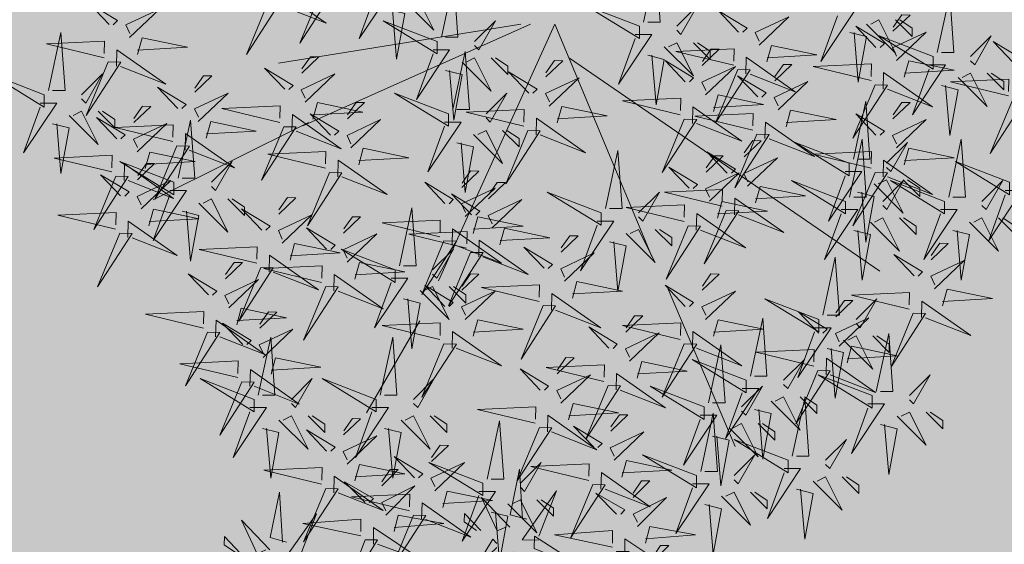
# Model space of a CAD drawing. Units: inches. Extents: x 1704 to 6393, y -157 to 1172.
# Tile 112 of 122: x 2688 to 2716, y 1003 to 1018. Entities that reach past the tile are written whole.
import ezdxf

# ---------------------------------------------------------------- set-up
doc = ezdxf.new("R2010")
doc.units = ezdxf.units.IN
doc.header["$MEASUREMENT"] = 0
doc.layers.add('A-ANNO-DIMS', color=7, linetype='Continuous', lineweight=13)
doc.layers.add('L-shrub', color=74, linetype='Continuous', lineweight=18)
doc.layers.add('L-HRDS-PATT', color=9, linetype='Continuous', lineweight=13, true_color=0xc5c1ba)
doc.styles.get("Standard").update_dxf_attribs({"font": 'arial.ttf'})
doc.dimstyles.get("Standard").update_dxf_attribs({"dimtxt": 6, "dimasz": 2, "dimexe": 0.18, "dimexo": 0.0625, "dimgap": 0.09, "dimtad": 0, "dimtih": 1, "dimtoh": 1, "dimdec": 1, "dimzin": 0, "dimdsep": 46, "dimlunit": 3, "dimtxsty": 'Standard', "dimblk": 'ARCHTICK', "dimcen": 0.09, "dimadec": 0, "dimazin": 0, "dimtfac": 1, "dimtdec": 1, "dimtofl": 0, "dimtmove": 0, "dimatfit": 3, "dimfxl": 1, "dimtolj": 1, "dimtzin": 0, "dimarcsym": 0})

# ---------------------------------------------------------------- blocks, each defined once
blk = doc.blocks.new('shrub3')
for p, q in [((-68.47, 143.52), (-106.19, 232.32)), ((68.94, 162.35), (98.58, 213.48)), ((-5.99, -2.5), (58.67, 140.12)), ((-14.08, 16.34), (-186.51, 134.74)), ((-5.99, -2.5), (-59.88, 126.66)), ((130.91, 52.02), (217.13, 95.08)), ((7.48, -2.5), (134.11, 54.01)), ((12.87, -2.5), (147.58, 19.03))]:
    blk.add_line(p, q)
for points in [[(29.32, 268.76), (20.08, 271.07), (24.7, 296.43), (27.01, 268.76)], [(72.58, 270.39), (84.86, 300.11), (65.67, 270.57), (72.58, 270.39)], [(-89.4, 264.53), (-98.64, 266.83), (-94.02, 292.2), (-91.71, 264.53)], [(36.24, 257.23), (27.01, 257.23), (45.48, 284.9), (36.24, 259.54)], [(121.34, 255.57), (133.62, 285.29), (114.43, 255.75), (121.34, 255.57)], [(-140.28, 256.06), (-149.52, 258.36), (-144.9, 283.73), (-142.59, 256.06)], [(-82.48, 253), (-91.71, 253), (-73.24, 280.67), (-82.48, 255.31)], [(-27.06, 253.45), (-14.78, 283.17), (-33.97, 253.63), (-27.06, 253.45)], [(20.08, 264.15), (3.92, 280.29), (13.16, 261.85), (17.78, 264.15)], [(68.03, 272.82), (67.8, 263.59), (40.6, 282.74), (65.73, 272.87)], [(-98.64, 259.92), (-114.8, 276.06), (-105.56, 257.61), (-100.94, 259.92)], [(-133.36, 244.53), (-142.59, 244.53), (-124.12, 272.2), (-133.36, 246.84)], [(3.92, 261.85), (-5.31, 271.07), (-5.31, 266.46), (1.62, 261.85)], [(-149.52, 251.45), (-165.68, 267.59), (-156.44, 249.14), (-151.83, 251.45)], [(-114.8, 257.61), (-124.03, 266.83), (-124.03, 262.22), (-117.11, 257.61)], [(-31.61, 255.88), (-31.84, 246.65), (-59.04, 265.8), (-33.91, 255.94)], [(56.33, 266.18), (53.8, 257.01), (28.56, 262.26), (56.27, 263.87)], [(74.83, 268.03), (106.93, 260.3), (74.6, 258.8), (74.77, 265.72)], [(116.79, 258), (116.56, 248.76), (89.36, 267.92), (114.49, 258.05)], [(-165.68, 249.14), (-174.91, 258.36), (-174.91, 253.75), (-167.99, 249.14)], [(13.16, 252.62), (1.62, 241.09), (10.85, 257.23), (13.16, 254.93)], [(33.94, 252.62), (63.95, 241.09), (33.94, 259.54), (33.94, 252.62)], [(-105.56, 248.39), (-117.11, 236.86), (-107.87, 253), (-105.56, 250.69)], [(-93.64, 226.42), (-102.88, 228.72), (-98.26, 254.08), (-95.95, 226.42)], [(-84.78, 248.39), (-54.77, 236.86), (-84.78, 255.31), (-84.78, 248.39)], [(60.71, 256.84), (44.17, 241.08), (62.84, 249.85), (60.65, 254.53)], [(123.59, 253.21), (155.69, 245.48), (123.36, 243.97), (123.53, 250.9)], [(-186.92, 220.06), (-196.16, 222.37), (-191.54, 247.73), (-189.23, 220.06)], [(-135.66, 239.92), (-105.65, 228.39), (-135.66, 246.84), (-135.66, 239.92)], [(-43.31, 249.24), (-45.84, 240.07), (-71.08, 245.32), (-43.37, 246.93)], [(-24.81, 251.09), (7.29, 243.36), (-25.04, 241.86), (-24.87, 248.78)], [(2.62, 221.69), (14.9, 251.41), (-4.29, 221.87), (2.62, 221.69)], [(31.63, 250.32), (24.7, 218.04), (22.39, 250.32), (29.32, 250.32)], [(72.06, 249.62), (83.3, 237.79), (67.4, 247.43), (69.76, 249.68)], [(105.09, 251.36), (102.56, 242.19), (77.32, 247.44), (105.04, 249.05)], [(88.68, 222.18), (79.44, 224.49), (84.06, 249.85), (86.37, 222.18)], [(156.52, 222.18), (147.29, 224.49), (151.9, 249.85), (154.21, 222.18)], [(-156.44, 239.92), (-167.99, 228.39), (-158.75, 244.53), (-156.44, 242.22)], [(-87.09, 246.08), (-94.02, 213.8), (-96.33, 246.08), (-89.4, 246.08)], [(-86.72, 214.89), (-95.95, 214.89), (-77.48, 242.56), (-86.72, 217.19)], [(109.47, 242.01), (92.93, 226.26), (111.6, 235.03), (109.41, 239.71)], [(-180, 208.53), (-189.23, 208.53), (-170.76, 236.2), (-180, 210.84)], [(-137.97, 237.61), (-144.9, 205.33), (-147.21, 237.61), (-140.28, 237.61)], [(-116.96, 211.59), (-126.2, 213.9), (-121.58, 239.26), (-119.27, 211.59)], [(-102.88, 221.8), (-119.04, 237.94), (-109.8, 219.5), (-105.18, 221.8)], [(-38.93, 239.9), (-55.47, 224.14), (-36.8, 232.91), (-38.99, 237.59)], [(62.61, 240.62), (53.16, 231.62), (57.77, 231.51), (62.55, 238.31)], [(95.61, 210.65), (86.37, 210.65), (104.84, 238.32), (95.61, 212.96)], [(163.45, 210.65), (154.21, 210.65), (172.68, 238.32), (163.45, 212.96)], [(-196.16, 215.45), (-212.32, 231.59), (-203.08, 213.15), (-198.47, 215.45)], [(-27.58, 232.68), (-16.34, 220.86), (-32.24, 230.49), (-29.88, 232.74)], [(-1.93, 224.12), (-2.16, 214.89), (-29.36, 234.04), (-4.23, 224.17)], [(79.44, 217.57), (63.28, 233.71), (72.52, 215.26), (77.14, 217.57)], [(120.82, 234.8), (132.06, 222.97), (116.16, 232.61), (118.52, 234.86)], [(147.29, 217.57), (131.13, 233.71), (140.36, 215.26), (144.98, 217.57)], [(-119.04, 219.5), (-128.27, 228.72), (-128.27, 224.11), (-121.35, 219.5)], [(-110.04, 200.06), (-119.27, 200.06), (-100.8, 227.73), (-110.04, 202.37)], [(-35.54, 198.4), (-23.26, 228.12), (-42.45, 198.58), (-35.54, 198.4)], [(63.28, 215.26), (54.05, 224.49), (54.05, 219.87), (60.98, 215.26)], [(111.37, 225.8), (101.92, 216.8), (106.53, 216.68), (111.31, 223.49)], [(131.13, 215.26), (121.89, 224.49), (121.89, 219.87), (128.82, 215.26)], [(167.98, 196.29), (180.26, 226), (161.07, 196.46), (167.98, 196.29)], [(-212.32, 213.15), (-221.55, 222.37), (-221.55, 217.76), (-214.63, 213.15)], [(-152.14, 189.93), (-139.86, 219.65), (-159.05, 190.11), (-152.14, 189.93)], [(-126.2, 206.98), (-142.36, 223.12), (-133.12, 204.68), (-128.5, 206.98)], [(-37.03, 223.68), (-46.48, 214.68), (-41.87, 214.57), (-37.09, 221.37)], [(4.87, 219.33), (36.97, 211.6), (4.64, 210.1), (4.81, 217.02)], [(-142.36, 204.68), (-151.59, 213.9), (-151.59, 209.29), (-144.67, 204.68)], [(-109.8, 210.27), (-121.35, 198.75), (-112.11, 214.89), (-109.8, 212.58)], [(-89.02, 210.27), (-59.01, 198.75), (-89.02, 217.19), (-89.02, 210.27)], [(-13.63, 217.48), (-16.16, 208.31), (-41.4, 213.56), (-13.69, 215.17)], [(-203.08, 203.92), (-214.63, 192.39), (-205.39, 208.53), (-203.08, 206.23)], [(-182.31, 203.92), (-152.29, 192.39), (-182.31, 210.84), (-182.31, 203.92)], [(-91.33, 207.97), (-98.26, 175.69), (-100.57, 207.97), (-93.64, 207.97)], [(-40.09, 200.83), (-40.32, 191.59), (-67.52, 210.75), (-42.39, 200.88)], [(-9.25, 208.13), (-25.79, 192.38), (-7.12, 201.15), (-9.31, 205.83)], [(72.52, 206.04), (60.98, 194.51), (70.21, 210.65), (72.52, 208.35)], [(93.3, 206.04), (123.31, 194.51), (93.3, 212.96), (93.3, 206.04)], [(140.36, 206.04), (128.82, 194.51), (138.05, 210.65), (140.36, 208.35)], [(163.43, 198.71), (163.2, 189.48), (136, 208.63), (161.13, 198.77)], [(161.14, 206.04), (191.15, 194.51), (161.14, 212.96), (161.14, 206.04)], [(-157.24, 177.72), (-166.48, 180.02), (-161.86, 205.38), (-159.55, 177.72)], [(-77.94, 175.11), (-65.66, 204.83), (-84.85, 175.28), (-77.94, 175.11)], [(55.62, 175.11), (67.9, 204.83), (48.71, 175.28), (55.62, 175.11)], [(90.99, 203.73), (84.06, 171.45), (81.75, 203.73), (88.68, 203.73)], [(158.83, 203.73), (151.9, 171.45), (149.59, 203.73), (156.52, 203.73)], [(-184.61, 201.62), (-191.54, 169.34), (-193.85, 201.62), (-186.92, 201.62)], [(-156.69, 192.36), (-156.92, 183.12), (-184.12, 202.28), (-159, 192.41)], [(-133.12, 195.45), (-144.67, 183.92), (-135.43, 200.06), (-133.12, 197.76)], [(-112.34, 195.45), (-82.33, 183.92), (-112.34, 202.37), (-112.34, 195.45)], [(2.1, 200.92), (13.34, 189.09), (-2.56, 198.73), (-0.2, 200.98)], [(187.06, 168.76), (199.34, 198.47), (180.15, 168.93), (187.06, 168.76)], [(-150.32, 166.19), (-159.55, 166.19), (-141.08, 193.86), (-150.32, 168.49)], [(-114.65, 193.15), (-121.58, 160.87), (-123.89, 193.15), (-116.96, 193.15)], [(-51.79, 194.19), (-54.32, 185.02), (-79.56, 190.27), (-51.85, 191.88)], [(-33.29, 196.04), (-1.19, 188.31), (-33.52, 186.81), (-33.35, 193.73)], [(-7.35, 191.92), (-16.8, 182.92), (-12.19, 182.81), (-7.41, 189.61)], [(151.73, 192.07), (149.2, 182.9), (123.96, 188.15), (151.68, 189.77)], [(170.23, 193.92), (202.33, 186.19), (170, 184.69), (170.17, 191.61)], [(-205.14, 158.17), (-192.86, 187.89), (-212.05, 158.35), (-205.14, 158.17)], [(-166.48, 173.1), (-182.64, 189.24), (-173.4, 170.8), (-168.79, 173.1)], [(-149.89, 187.57), (-117.79, 179.84), (-150.12, 178.34), (-149.95, 185.26)], [(-82.49, 177.53), (-82.72, 168.3), (-109.92, 187.46), (-84.79, 177.59)], [(51.07, 177.53), (50.84, 168.3), (23.64, 187.46), (48.77, 177.59)], [(-168.39, 185.72), (-170.92, 176.55), (-196.16, 181.8), (-168.45, 183.41)], [(-47.41, 184.84), (-63.95, 169.09), (-45.28, 177.86), (-47.47, 182.54)], [(0.5, 153.94), (12.78, 183.65), (-6.41, 154.11), (0.5, 153.94)], [(156.11, 182.73), (139.57, 166.97), (158.24, 175.74), (156.05, 180.42)], [(182.51, 171.18), (182.28, 161.95), (155.08, 181.11), (180.21, 171.24)], [(-182.64, 170.8), (-191.87, 180.02), (-191.87, 175.41), (-184.95, 170.8)], [(-164.01, 176.37), (-180.55, 160.62), (-161.88, 169.39), (-164.07, 174.07)], [(-36.06, 177.63), (-24.82, 165.8), (-40.72, 175.44), (-38.36, 177.69)], [(78.08, 150.19), (68.84, 152.49), (73.46, 177.86), (75.77, 150.19)], [(167.46, 175.51), (178.7, 163.69), (162.8, 173.32), (165.16, 175.57)], [(-209.69, 160.6), (-209.92, 151.36), (-237.12, 170.52), (-212, 160.65)], [(-94.19, 170.9), (-96.72, 161.73), (-121.96, 166.98), (-94.25, 168.59)], [(-75.69, 172.75), (-43.59, 165.01), (-75.92, 163.51), (-75.75, 170.44)], [(39.37, 170.9), (36.84, 161.73), (11.6, 166.98), (39.31, 168.59)], [(57.87, 172.75), (89.97, 165.01), (57.64, 163.51), (57.81, 170.44)], [(121.34, 143.35), (133.62, 173.06), (114.43, 143.52), (121.34, 143.35)], [(-173.4, 161.57), (-184.95, 150.05), (-175.71, 166.19), (-173.4, 163.88)], [(-152.66, 169.16), (-141.42, 157.33), (-157.33, 166.97), (-154.96, 169.22)], [(-152.62, 161.57), (-122.61, 150.05), (-152.62, 168.49), (-152.62, 161.57)], [(-45.51, 168.63), (-54.96, 159.63), (-50.35, 159.51), (-45.57, 166.32)], [(-4.05, 156.36), (-4.28, 147.13), (-31.48, 166.28), (-6.35, 156.42)], [(85.01, 138.66), (75.77, 138.66), (94.24, 166.33), (85.01, 140.97)], [(170.81, 164.55), (168.28, 155.37), (143.04, 160.62), (170.76, 162.24)], [(158.01, 166.51), (148.56, 157.51), (153.17, 157.4), (157.96, 164.21)], [(189.31, 166.39), (221.41, 158.66), (189.08, 157.16), (189.25, 164.09)], [(-162.11, 160.16), (-171.56, 151.16), (-166.95, 151.04), (-162.17, 157.85)], [(-154.93, 159.27), (-161.86, 126.99), (-164.17, 159.27), (-157.24, 159.27)], [(-89.81, 161.55), (-106.35, 145.8), (-87.68, 154.57), (-89.87, 159.24)], [(43.75, 161.55), (27.21, 145.8), (45.88, 154.57), (43.69, 159.24)], [(68.84, 145.58), (52.68, 161.72), (61.92, 143.27), (66.54, 145.58)], [(157.38, 132.76), (169.66, 162.48), (150.47, 132.94), (157.38, 132.76)], [(-221.39, 153.96), (-223.93, 144.79), (-249.17, 150.04), (-221.45, 151.65)], [(-202.89, 155.81), (-170.79, 148.07), (-203.12, 146.57), (-202.95, 153.5)], [(-78.46, 154.34), (-67.22, 142.51), (-83.13, 152.15), (-80.76, 154.4)], [(40.78, 124.29), (53.06, 154.01), (33.87, 124.47), (40.78, 124.29)], [(55.1, 154.34), (66.34, 142.51), (50.44, 152.15), (52.8, 154.4)], [(116.79, 145.77), (116.56, 136.54), (89.36, 155.7), (114.49, 145.83)], [(175.19, 155.2), (158.65, 139.45), (177.32, 148.22), (175.13, 152.89)], [(-15.75, 149.73), (-18.28, 140.55), (-43.52, 145.8), (-15.81, 147.42)], [(2.75, 151.57), (34.85, 143.84), (2.52, 142.34), (2.69, 149.26)], [(52.68, 143.27), (43.45, 152.49), (43.45, 147.88), (50.38, 143.27)], [(186.54, 147.99), (197.78, 136.16), (181.88, 145.8), (184.24, 148.05)], [(-217.01, 144.61), (-233.55, 128.86), (-214.88, 137.63), (-217.07, 142.31)], [(-87.91, 145.34), (-97.36, 136.34), (-92.75, 136.22), (-87.97, 143.03)], [(-36.4, 118.43), (-45.64, 120.73), (-41.02, 146.1), (-38.71, 118.43)], [(45.65, 145.34), (36.2, 136.34), (40.81, 136.22), (45.59, 143.03)], [(55.62, 117.94), (67.9, 147.66), (48.71, 118.11), (55.62, 117.94)], [(152.83, 135.19), (152.6, 125.95), (125.4, 145.11), (150.53, 135.24)], [(235.82, 113.71), (248.1, 143.42), (228.91, 113.88), (235.82, 113.71)], [(-227.2, 112.08), (-236.44, 114.38), (-231.82, 139.75), (-229.51, 112.08)], [(-205.66, 137.4), (-194.42, 125.57), (-210.33, 135.21), (-207.96, 137.46)], [(-172.08, 112.08), (-181.32, 114.38), (-176.7, 139.75), (-174.39, 112.08)], [(-80.06, 109.47), (-67.78, 139.19), (-86.97, 109.65), (-80.06, 109.47)], [(-11.37, 140.38), (-27.91, 124.63), (-9.24, 133.4), (-11.43, 138.07)], [(61.92, 134.05), (50.38, 122.52), (59.61, 138.66), (61.92, 136.35)], [(105.09, 139.14), (102.56, 129.96), (77.32, 135.21), (105.04, 136.83)], [(82.7, 134.05), (112.71, 122.52), (82.7, 140.97), (82.7, 134.05)], [(123.59, 140.98), (155.69, 133.25), (123.36, 131.75), (123.53, 138.68)], [(177.09, 138.99), (167.64, 129.99), (172.25, 129.87), (177.04, 136.68)], [(-29.48, 106.9), (-38.71, 106.9), (-20.24, 134.57), (-29.48, 109.2)], [(-0.02, 133.17), (11.22, 121.34), (-4.68, 130.97), (-2.32, 133.22)], [(36.23, 126.72), (36, 117.49), (8.8, 136.64), (33.93, 126.77)], [(80.39, 131.74), (73.46, 99.46), (71.15, 131.74), (78.08, 131.74)], [(-263.24, 101.49), (-272.48, 103.79), (-267.86, 129.16), (-265.55, 101.49)], [(-220.28, 100.55), (-229.51, 100.55), (-211.04, 128.22), (-220.28, 102.85)], [(-215.11, 128.4), (-224.56, 119.4), (-219.95, 119.28), (-215.17, 126.09)], [(-165.16, 100.55), (-174.39, 100.55), (-155.92, 128.22), (-165.16, 102.85)], [(-101.26, 101), (-88.98, 130.72), (-108.17, 101.18), (-101.26, 101)], [(-45.64, 113.82), (-61.8, 129.96), (-52.56, 111.51), (-47.94, 113.82)], [(51.07, 120.36), (50.84, 111.13), (23.64, 130.29), (48.77, 120.42)], [(109.47, 129.79), (92.93, 114.04), (111.6, 122.81), (109.41, 127.48)], [(141.13, 128.55), (138.6, 119.38), (113.36, 124.63), (141.08, 126.24)], [(159.63, 130.4), (191.73, 122.67), (159.4, 121.17), (159.57, 128.09)], [(201.04, 101.49), (191.81, 103.79), (196.42, 129.16), (198.73, 101.49)], [(231.27, 116.13), (231.04, 106.9), (203.84, 126.05), (228.97, 116.19)], [(-236.44, 107.46), (-252.6, 123.6), (-243.36, 105.16), (-238.75, 107.46)], [(-181.32, 107.46), (-197.48, 123.6), (-188.24, 105.16), (-183.63, 107.46)], [(-84.61, 111.9), (-84.84, 102.66), (-112.04, 121.82), (-86.91, 111.95)], [(-61.8, 111.51), (-71.03, 120.73), (-71.03, 116.12), (-64.1, 111.51)], [(-9.47, 124.17), (-18.92, 115.16), (-14.31, 115.05), (-9.53, 121.86)], [(43.03, 121.93), (75.13, 114.2), (42.8, 112.7), (42.97, 119.62)], [(120.82, 122.58), (132.06, 110.75), (116.16, 120.39), (118.52, 122.64)], [(-256.32, 89.96), (-265.55, 89.96), (-247.08, 117.63), (-256.32, 92.27)], [(-174.2, 90.9), (-183.44, 93.21), (-178.82, 118.57), (-176.51, 90.9)], [(24.53, 120.08), (22, 110.91), (-3.24, 116.16), (24.47, 117.77)], [(57.87, 115.58), (89.97, 107.84), (57.64, 106.34), (57.81, 113.27)], [(145.51, 119.2), (128.97, 103.45), (147.64, 112.22), (145.45, 116.9)], [(207.97, 89.96), (198.73, 89.96), (217.2, 117.63), (207.97, 92.27)], [(-272.48, 96.88), (-288.64, 113.02), (-279.4, 94.57), (-274.79, 96.88)], [(-252.6, 105.16), (-261.83, 114.38), (-261.83, 109.77), (-254.91, 105.16)], [(-197.48, 105.16), (-206.71, 114.38), (-206.71, 109.77), (-199.79, 105.16)], [(-183.94, 79.83), (-171.66, 109.54), (-190.85, 80), (-183.94, 79.83)], [(-105.81, 103.43), (-106.04, 94.19), (-133.24, 113.35), (-108.11, 103.48)], [(39.37, 113.73), (36.84, 104.56), (11.6, 109.81), (39.31, 111.42)], [(28.91, 110.73), (12.37, 94.98), (31.04, 103.75), (28.85, 108.43)], [(111.37, 113.58), (101.92, 104.58), (106.53, 104.46), (111.31, 111.27)], [(119.22, 79.83), (131.5, 109.54), (112.31, 80), (119.22, 79.83)], [(156.86, 111.99), (168.1, 100.16), (152.2, 109.8), (154.56, 112.05)], [(191.81, 96.88), (175.65, 113.02), (184.88, 94.57), (189.5, 96.88)], [(219.57, 109.49), (217.04, 100.32), (191.8, 105.57), (219.52, 107.19)], [(237.94, 81.95), (250.22, 111.66), (231.03, 82.12), (237.94, 81.95)], [(238.07, 111.34), (270.17, 103.61), (237.84, 102.11), (238.01, 109.03)], [(-167.28, 79.37), (-176.51, 79.37), (-158.04, 107.04), (-167.28, 81.68)], [(-96.31, 105.26), (-98.84, 96.09), (-124.08, 101.34), (-96.37, 102.95)], [(-77.81, 107.11), (-45.71, 99.37), (-78.04, 97.87), (-77.87, 104.8)], [(-52.56, 102.29), (-64.1, 90.76), (-54.87, 106.9), (-52.56, 104.59)], [(-31.78, 102.29), (-1.77, 90.76), (-31.78, 109.2), (-31.78, 102.29)], [(43.75, 104.38), (27.21, 88.63), (45.88, 97.4), (43.69, 102.07)], [(-288.64, 94.57), (-297.87, 103.79), (-297.87, 99.18), (-290.95, 94.57)], [(-243.36, 95.94), (-254.91, 84.41), (-245.67, 100.55), (-243.36, 98.24)], [(-222.59, 95.94), (-192.57, 84.41), (-222.59, 102.85), (-222.59, 95.94)], [(-188.24, 95.94), (-199.79, 84.41), (-190.55, 100.55), (-188.24, 98.24)], [(-183.44, 86.29), (-199.6, 102.43), (-190.36, 83.98), (-185.75, 86.29)], [(-167.46, 95.94), (-137.45, 84.41), (-167.46, 102.85), (-167.46, 95.94)], [(-99.01, 98.64), (-66.91, 90.91), (-99.24, 89.41), (-99.07, 96.33)], [(-34.09, 99.98), (-41.02, 67.7), (-43.33, 99.98), (-36.4, 99.98)], [(40.26, 103.52), (51.5, 91.69), (35.6, 101.33), (37.96, 103.58)], [(147.41, 102.99), (137.96, 93.99), (142.57, 93.88), (147.36, 100.68)], [(175.65, 94.57), (166.41, 103.79), (166.41, 99.18), (173.34, 94.57)], [(223.95, 100.15), (207.41, 84.4), (226.08, 93.17), (223.89, 97.84)], [(-224.89, 93.63), (-231.82, 61.35), (-234.13, 93.63), (-227.2, 93.63)], [(-199.6, 83.98), (-208.83, 93.21), (-208.83, 88.6), (-201.91, 83.98)], [(-169.77, 93.63), (-176.7, 61.35), (-179.01, 93.63), (-172.08, 93.63)], [(-117.51, 96.79), (-120.04, 87.62), (-145.28, 92.87), (-117.57, 94.48)], [(-91.93, 95.91), (-108.47, 80.16), (-89.8, 88.93), (-91.99, 93.61)], [(30.81, 94.52), (21.36, 85.52), (25.97, 85.41), (30.75, 92.21)], [(55.1, 97.17), (66.34, 85.34), (50.44, 94.98), (52.8, 97.23)], [(204.02, 65.01), (216.3, 94.72), (197.11, 65.18), (204.02, 65.01)], [(233.39, 84.37), (233.16, 75.14), (205.96, 94.29), (231.09, 84.43)], [(-279.4, 85.35), (-290.95, 73.82), (-281.71, 89.96), (-279.4, 87.65)], [(-258.63, 85.35), (-228.61, 73.82), (-258.63, 92.27), (-258.63, 85.35)], [(-188.49, 82.25), (-188.72, 73.02), (-215.92, 92.18), (-190.8, 82.31)], [(-118.22, 58.65), (-105.94, 88.37), (-125.13, 58.83), (-118.22, 58.65)], [(-80.58, 88.7), (-69.34, 76.87), (-85.25, 86.51), (-82.88, 88.76)], [(45.65, 88.17), (36.2, 79.17), (40.81, 79.05), (45.59, 85.86)], [(48.4, 63.38), (39.16, 65.68), (43.78, 91.04), (46.09, 63.38)], [(114.67, 82.25), (114.44, 73.02), (87.24, 92.18), (112.37, 82.31)], [(184.88, 85.35), (173.34, 73.82), (182.57, 89.96), (184.88, 87.65)], [(205.66, 85.35), (235.67, 73.82), (205.66, 92.27), (205.66, 85.35)], [(235.3, 92.94), (246.54, 81.11), (230.64, 90.74), (233, 92.99)], [(-260.93, 83.04), (-267.86, 50.76), (-270.17, 83.04), (-263.24, 83.04)], [(-113.13, 87.44), (-129.67, 71.69), (-111, 80.46), (-113.19, 85.14)], [(8.98, 56.54), (21.26, 86.25), (2.07, 56.71), (8.98, 56.54)], [(144.66, 54.42), (156.94, 84.13), (137.75, 54.59), (144.66, 54.42)], [(203.35, 83.04), (196.42, 50.76), (194.11, 83.04), (201.04, 83.04)], [(225.85, 83.93), (216.4, 74.93), (221.01, 74.82), (225.8, 81.63)], [(-190.36, 74.76), (-201.91, 63.23), (-192.67, 79.37), (-190.36, 77.07)], [(-181.69, 77.46), (-149.59, 69.73), (-181.92, 68.23), (-181.75, 75.15)], [(-169.58, 74.76), (-139.57, 63.23), (-169.58, 81.68), (-169.58, 74.76)], [(-101.78, 80.23), (-90.54, 68.4), (-106.45, 78.04), (-104.08, 80.29)], [(-90.03, 79.7), (-99.48, 70.7), (-94.87, 70.58), (-90.09, 77.39)], [(-77.94, 50.18), (-65.66, 79.9), (-84.85, 50.36), (-77.94, 50.18)], [(55.33, 51.85), (46.09, 51.85), (64.56, 79.52), (55.33, 54.15)], [(121.47, 77.46), (153.57, 69.73), (121.24, 68.23), (121.41, 75.15)], [(199.47, 67.43), (199.24, 58.2), (172.04, 77.35), (197.17, 67.49)], [(221.69, 77.73), (219.16, 68.56), (193.92, 73.81), (221.64, 75.43)], [(240.19, 79.58), (272.29, 71.85), (239.96, 70.35), (240.13, 77.27)], [(273.12, 52.79), (263.89, 55.09), (268.5, 80.46), (270.81, 52.79)], [(-200.19, 75.62), (-202.73, 66.44), (-227.97, 71.69), (-200.25, 73.31)], [(-171.89, 72.46), (-178.82, 40.17), (-181.13, 72.46), (-174.2, 72.46)], [(-111.23, 71.23), (-120.68, 62.23), (-116.07, 62.11), (-111.29, 68.92)], [(39.16, 58.76), (23, 74.9), (32.24, 56.46), (36.86, 58.76)], [(102.97, 75.62), (100.44, 66.44), (75.2, 71.69), (102.92, 73.31)], [(-260.26, 39.6), (-247.98, 69.31), (-267.17, 39.77), (-260.26, 39.6)], [(-195.81, 66.27), (-212.35, 50.52), (-193.68, 59.29), (-195.87, 63.96)], [(-122.77, 61.08), (-123, 51.85), (-150.2, 71), (-125.08, 61.14)], [(4.43, 58.96), (4.2, 49.73), (-23, 68.88), (2.13, 59.02)], [(23, 56.46), (13.77, 65.68), (13.77, 61.07), (20.7, 56.46)], [(107.35, 66.27), (90.81, 50.52), (109.48, 59.29), (107.29, 63.96)], [(140.11, 56.84), (139.88, 47.61), (112.68, 66.77), (137.81, 56.9)], [(226.07, 68.39), (209.53, 52.64), (228.2, 61.41), (226.01, 66.08)], [(280.05, 41.26), (270.81, 41.26), (289.28, 68.93), (280.05, 43.57)], [(-183.94, 31.13), (-171.66, 60.84), (-190.85, 31.3), (-183.94, 31.13)], [(-82.49, 52.61), (-82.72, 43.38), (-109.92, 62.53), (-84.79, 52.67)], [(187.77, 60.79), (185.24, 51.62), (160, 56.87), (187.72, 58.49)], [(206.27, 62.64), (238.37, 54.91), (206.04, 53.41), (206.21, 60.33)], [(237.42, 61.17), (248.66, 49.35), (232.76, 58.98), (235.12, 61.23)], [(263.89, 48.18), (247.73, 64.32), (256.96, 45.87), (261.58, 48.18)], [(-220.84, 31.61), (-230.08, 33.92), (-225.46, 59.28), (-223.15, 31.61)], [(-184.46, 59.06), (-173.22, 47.23), (-189.13, 56.86), (-186.76, 59.12)], [(-115.97, 56.29), (-83.87, 48.56), (-116.2, 47.06), (-116.03, 53.98)], [(118.7, 59.06), (129.94, 47.23), (114.04, 56.86), (116.4, 59.12)], [(247.73, 45.87), (238.49, 55.09), (238.49, 50.48), (245.42, 45.87)], [(-264.81, 42.02), (-265.04, 32.79), (-292.24, 51.95), (-267.12, 42.08)], [(-193.91, 50.06), (-203.36, 41.06), (-198.75, 40.94), (-193.97, 47.75)], [(-134.47, 54.44), (-137, 45.27), (-162.24, 50.52), (-134.53, 52.13)], [(-107.62, 22.66), (-95.34, 52.37), (-114.53, 22.83), (-107.62, 22.66)], [(-7.27, 52.33), (-9.8, 43.15), (-35.04, 48.4), (-7.33, 50.02)], [(11.23, 54.17), (43.33, 46.44), (11, 44.94), (11.17, 51.86)], [(32.24, 47.24), (20.7, 35.71), (29.93, 51.85), (32.24, 49.54)], [(54.76, 23.15), (45.52, 25.45), (50.14, 50.81), (52.45, 23.15)], [(53.02, 47.24), (83.03, 35.71), (53.02, 54.15), (53.02, 47.24)], [(109.25, 50.06), (99.8, 41.06), (104.41, 40.94), (109.19, 47.75)], [(128.41, 50.21), (125.88, 41.03), (100.64, 46.28), (128.36, 47.9)], [(146.91, 52.05), (179.01, 44.32), (146.68, 42.82), (146.85, 49.75)], [(192.15, 51.45), (175.61, 35.7), (194.28, 44.47), (192.09, 49.14)], [(227.97, 52.17), (218.52, 43.17), (223.13, 43.06), (227.92, 49.87)], [(-213.92, 20.09), (-223.15, 20.09), (-204.68, 47.76), (-213.92, 22.39)], [(-130.09, 45.1), (-146.63, 29.34), (-127.96, 38.11), (-130.15, 42.79)], [(-94.19, 45.97), (-96.72, 36.8), (-121.96, 42.05), (-94.25, 43.67)], [(-75.69, 47.82), (-43.59, 40.09), (-75.92, 38.59), (-75.75, 45.51)], [(50.71, 44.93), (43.78, 12.65), (41.47, 44.93), (48.4, 44.93)], [(203.5, 44.24), (214.74, 32.41), (198.84, 42.04), (201.2, 44.29)], [(242.18, 18.42), (254.46, 48.14), (235.27, 18.6), (242.18, 18.42)], [(-230.08, 27), (-246.24, 43.14), (-237, 24.7), (-232.39, 27)], [(-188.49, 33.55), (-188.72, 24.32), (-215.92, 43.48), (-190.8, 33.61)], [(-57.6, 14.68), (-66.84, 16.98), (-62.22, 42.34), (-59.91, 14.68)], [(-2.89, 42.98), (-19.43, 27.23), (-0.76, 36), (-2.95, 40.67)], [(61.69, 11.62), (52.45, 11.62), (70.92, 39.29), (61.69, 13.92)], [(132.79, 40.86), (116.25, 25.11), (134.92, 33.88), (132.73, 38.55)], [(256.96, 36.65), (245.42, 25.12), (254.65, 41.26), (256.96, 38.95)], [(277.74, 36.65), (307.75, 25.12), (277.74, 43.57), (277.74, 36.65)], [(-276.51, 35.39), (-279.05, 26.21), (-304.29, 31.46), (-276.57, 33.08)], [(-258.01, 37.23), (-225.91, 29.5), (-258.24, 28), (-258.07, 34.92)], [(-246.24, 24.7), (-255.47, 33.92), (-255.47, 29.31), (-248.55, 24.7)], [(-112.17, 25.08), (-112.4, 15.85), (-139.6, 35.01), (-114.47, 25.14)], [(-118.74, 37.88), (-107.5, 26.06), (-123.41, 35.69), (-121.04, 37.94)], [(-89.81, 36.63), (-106.35, 20.87), (-87.68, 29.64), (-89.87, 34.32)], [(8.46, 35.77), (19.7, 23.94), (3.8, 33.57), (6.16, 35.82)], [(45.52, 18.53), (29.36, 34.67), (38.6, 16.23), (43.22, 18.53)], [(144.14, 33.65), (155.38, 21.82), (139.48, 31.46), (141.84, 33.71)], [(194.05, 35.23), (184.6, 26.23), (189.21, 26.12), (194, 32.93)], [(275.43, 34.34), (268.5, 2.06), (266.19, 34.34), (273.12, 34.34)], [(-181.69, 28.76), (-149.59, 21.03), (-181.92, 19.53), (-181.75, 26.45)], [(-169.96, 1.97), (-179.2, 4.28), (-174.58, 29.64), (-172.27, 1.97)], [(-128.19, 28.88), (-137.64, 19.88), (-133.03, 19.77), (-128.25, 26.57)], [(-78.46, 29.41), (-67.22, 17.59), (-83.13, 27.22), (-80.76, 29.47)], [(-50.68, 3.15), (-59.91, 3.15), (-41.44, 30.82), (-50.68, 5.45)], [(237.63, 20.85), (237.4, 11.62), (210.2, 30.77), (235.33, 20.91)], [(-272.13, 26.04), (-288.67, 10.29), (-270, 19.06), (-272.19, 23.73)], [(-200.19, 26.92), (-202.73, 17.74), (-227.97, 22.99), (-200.25, 24.61)], [(-216.23, 15.47), (-186.21, 3.95), (-216.23, 22.39), (-216.23, 15.47)], [(-66.84, 10.06), (-83, 26.2), (-73.76, 7.76), (-69.14, 10.06)], [(-0.99, 26.77), (-10.44, 17.76), (-5.83, 17.65), (-1.05, 24.46)], [(29.36, 16.23), (20.13, 25.45), (20.13, 20.84), (27.06, 16.23)], [(134.69, 24.65), (125.24, 15.65), (129.85, 15.53), (134.63, 22.34)], [(-260.78, 18.83), (-249.54, 7), (-265.45, 16.63), (-263.08, 18.88)], [(-237, 15.47), (-248.55, 3.95), (-239.31, 20.09), (-237, 17.78)], [(-195.81, 17.57), (-212.35, 1.82), (-193.68, 10.59), (-195.87, 15.26)], [(-163.04, -9.56), (-172.27, -9.56), (-153.8, 18.11), (-163.04, -7.25)], [(-123.87, 18.45), (-126.4, 9.27), (-151.64, 14.52), (-123.93, 16.14)], [(-105.37, 20.29), (-73.27, 12.56), (-105.6, 11.06), (-105.43, 17.99)], [(-87.91, 20.41), (-97.36, 11.41), (-92.75, 11.3), (-87.97, 18.11)], [(-83, 7.76), (-92.23, 16.98), (-92.23, 12.37), (-85.3, 7.76)], [(86.56, -10.73), (77.32, -8.43), (81.94, 16.94), (84.25, -10.73)], [(-218.53, 13.17), (-225.46, -19.11), (-227.77, 13.17), (-220.84, 13.17)], [(-179.2, -2.64), (-195.36, 13.5), (-186.12, -4.95), (-181.51, -2.64)], [(38.6, 7), (27.06, -4.52), (36.29, 11.62), (38.6, 9.31)], [(59.38, 7), (89.39, -4.52), (59.38, 13.92), (59.38, 7)], [(153.14, -15.45), (165.42, 14.26), (146.23, -15.28), (153.14, -15.45)], [(225.93, 14.21), (223.4, 5.04), (198.16, 10.29), (225.88, 11.9)], [(244.43, 16.06), (276.53, 8.33), (244.2, 6.83), (244.37, 13.75)], [(-270.23, 9.83), (-279.68, 0.83), (-275.07, 0.71), (-270.29, 7.52)], [(-184.46, 10.36), (-173.22, -1.47), (-189.13, 8.16), (-186.76, 10.41)], [(-119.49, 9.1), (-136.03, -6.65), (-117.36, 2.12), (-119.55, 6.79)], [(123.46, -21.81), (135.74, 7.91), (116.55, -21.63), (123.46, -21.81)], [(-195.36, -4.95), (-204.59, 4.28), (-204.59, -0.33), (-197.67, -4.95)], [(-193.91, 1.36), (-203.36, -7.64), (-198.75, -7.76), (-193.97, -0.95)], [(-108.14, 1.89), (-96.9, -9.94), (-112.81, -0.3), (-110.44, 1.95)], [(-73.76, -1.46), (-85.3, -12.99), (-76.07, 3.15), (-73.76, 0.84)], [(-52.98, -1.46), (-22.97, -12.99), (-52.98, 5.45), (-52.98, -1.46)], [(57.07, 4.7), (50.14, -27.58), (47.83, 4.7), (54.76, 4.7)], [(77.32, -15.34), (61.16, 0.8), (70.4, -17.65), (75.02, -15.34)], [(93.49, -22.26), (84.25, -22.26), (102.72, 5.41), (93.49, -19.96)], [(230.31, 4.87), (213.77, -10.89), (232.44, -2.12), (230.25, 2.56)], [(-55.29, -3.77), (-62.22, -36.05), (-64.53, -3.77), (-57.6, -3.77)], [(148.59, -13.03), (148.36, -22.26), (121.16, -3.11), (146.29, -12.97)], [(241.66, -2.35), (252.9, -14.18), (237, -4.54), (239.36, -2.29)], [(-269.6, -38.26), (-278.84, -35.95), (-274.22, -10.59), (-271.91, -38.26)], [(-278.84, -42.87), (-295, -26.73), (-285.76, -45.18), (-281.15, -42.87)], [(-262.68, -49.79), (-271.91, -49.79), (-253.44, -22.12), (-262.68, -47.48)], [(-295, -45.18), (-304.23, -35.95), (-304.23, -40.56), (-297.31, -45.18)], [(-264.99, -54.4), (-234.97, -65.93), (-264.99, -47.48), (-264.99, -54.4)], [(-285.76, -54.4), (-297.31, -65.93), (-288.07, -49.79), (-285.76, -52.09)], [(-267.29, -56.71), (-274.22, -88.99), (-276.53, -56.71), (-269.6, -56.71)], [(-252.09, -91.37), (-252.32, -100.61), (-279.52, -81.45), (-254.4, -91.32)], [(-263.79, -98.01), (-266.33, -107.18), (-291.57, -101.93), (-263.85, -100.32)], [(-259.41, -107.36), (-275.95, -123.11), (-257.28, -114.34), (-259.47, -109.66)], [(-257.51, -123.57), (-266.96, -132.57), (-262.35, -132.69), (-257.57, -125.88)]]:
    blk.add_lwpolyline(points)
blk = doc.blocks.new('_ArchTick')
at = {"color": 0, "linetype": 'ByBlock', "const_width": 0.15}
blk.add_lwpolyline([(-0.5, -0.5), (0.5, 0.5)], dxfattribs=at)
blk = doc.blocks.new('*D95')
at = {"layer": 'A-ANNO-DIMS', "color": 0, "lineweight": -2, "transparency": 16777216}
for p, q in [((2605.349, 895.275), (2605.349, 1105.287)), ((2723.349, 895.275), (2723.349, 1105.287)), ((2605.349, 1105.107), (2657.907, 1105.107)), ((2723.349, 1105.107), (2670.791, 1105.107))]:
    blk.add_line(p, q, dxfattribs=at)
at = {"layer": 'Defpoints', "color": 0, "lineweight": -3, "transparency": 16777216}
for p in [(2723.349, 1105.107), (2605.349, 895.213), (2723.349, 895.213)]:
    blk.add_point(p, dxfattribs=at)
at = {"layer": 'A-ANNO-DIMS', "color": 0, "lineweight": -2, "transparency": 16777216, "xscale": 2, "yscale": 2, "zscale": 2, "rotation": 180}
blk.add_blockref('_ArchTick', (2605.349, 1105.107), dxfattribs=at)
at = {"layer": 'A-ANNO-DIMS', "color": 0, "lineweight": -2, "transparency": 16777216, "xscale": 2, "yscale": 2, "zscale": 2}
blk.add_blockref('_ArchTick', (2723.349, 1105.107), dxfattribs=at)
at = {"layer": 'A-ANNO-DIMS', "color": 0, "transparency": 16777216, "insert": (2664.349, 1105.107), "char_height": 6, "attachment_point": 5}
blk.add_mtext('\\A1;118', dxfattribs=at)

msp = doc.modelspace()

# ---------------------------------------------------------------- hatches: boundary and pattern name
at = {"layer": 'L-HRDS-PATT', "transparency": 33554661}
h = msp.add_hatch(color=256, dxfattribs=at)
h.dxf.hatch_style = 1
h.paths.add_polyline_path([(2719.349, 1033.213), (2664.349, 1033.213), (2664.349, 895.213), (2719.349, 895.213)])
h.paths.add_polyline_path([(2719.349, 895.213), (2664.349, 895.213), (2605.349, 895.213), (2605.349, 872.213), (2719.349, 872.213)])
h.paths.add_polyline_path([(2719.349, 872.213), (2605.349, 872.213), (2605.349, 854.213), (2601.349, 854.213, -0.121066), (2618.034, 850.113), (2618.05, 850.14), (2619.349, 849.39), (2601.349, 818.213), (2605.349, 818.213), (2605.349, 794.213), (2605.349, 754.213), (2631.349, 754.213), (2631.349, 716.213), (2719.349, 716.213)])

# ---------------------------------------------------------------- block references
at = {"layer": 'L-shrub', "xscale": 0.0510581485411622, "yscale": 0.0510581485411622, "zscale": 0.0510581485411622}
for p, rotation in [((2703.343, 1017.291), 180), ((2701.044, 989.25), 269.9999999999999)]:
    msp.add_blockref('shrub3', p, dxfattribs=dict(at, rotation=rotation))

# ---------------------------------------------------------------- dimensions: what is measured, and where the dimension line sits
at = {"layer": 'A-ANNO-DIMS'}
dim = msp.add_linear_dim(base=(2723.349, 1105.107), p1=(2605.349, 895.213), p2=(2723.349, 895.213), dimstyle='Standard', override={"dimdec": 0, "dimlfac": 1, "dimrnd": 0, "dimzin": 0, "dimdsep": 46, "dimlunit": 2}, dxfattribs=at)
dim.commit()
dim.dimension.update_dxf_attribs({"geometry": '*D95', "text_midpoint": (2664.349, 1105.107)})

doc.saveas('drawing.dxf')
